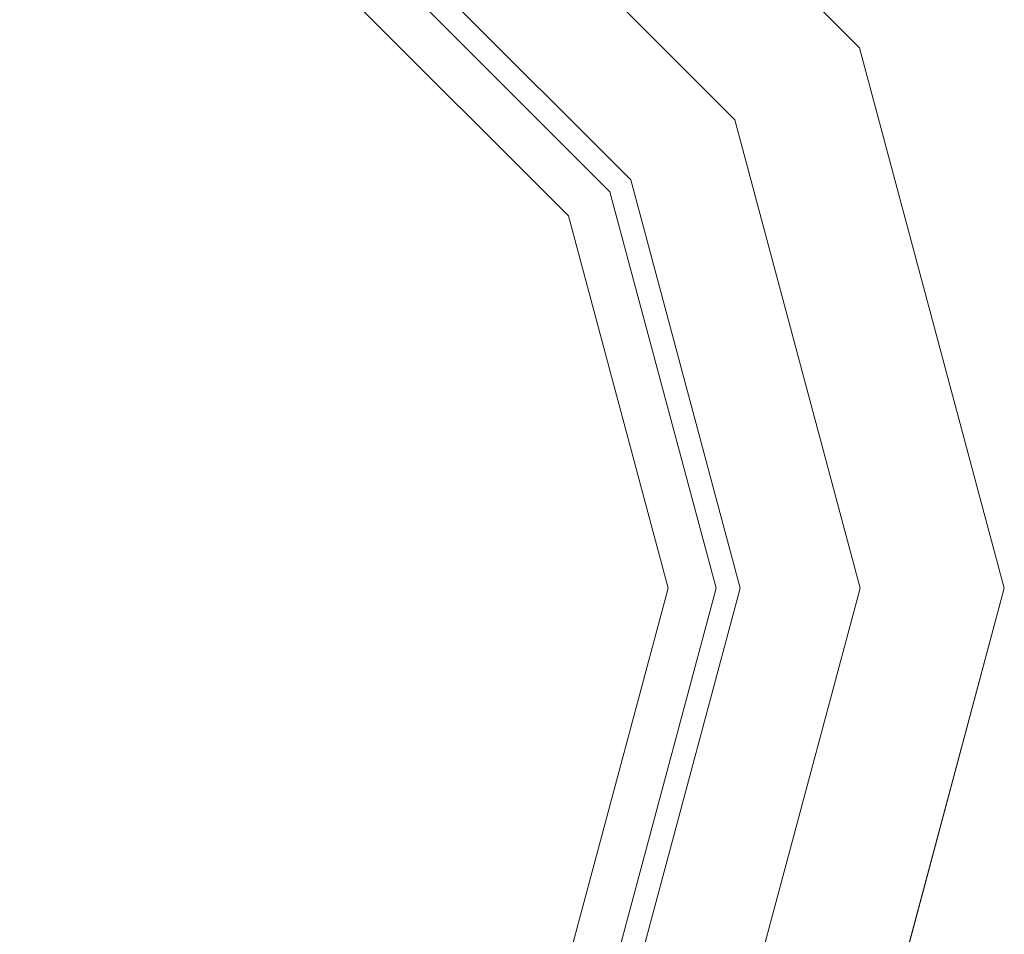
# Model space of a CAD drawing. Units: inches. Extents: x 375 to 1122, y 27 to 1069.
# Tile 24 of 155: x 713.046 to 718.094, y 275.466 to 280.154. Entities that reach past the tile are written whole.
import ezdxf

# ---------------------------------------------------------------- set-up
doc = ezdxf.new("R2010")
doc.units = ezdxf.units.IN
doc.layers.add('Furniture', color=30, linetype='Continuous', lineweight=18)

# ---------------------------------------------------------------- blocks, each defined once
blk = doc.blocks.new('A$C403C54AD')
at = {"linetype": 'ByBlock'}
for points, invisible_edges in [([(1.72651, 0.82864, -0.00874), (1.72651, 0.81017, -0.00874), (1.66648, 0.79408, -0.00874), (1.65725, 0.81008, -0.00874)], 5), ([(1.72651, 0.79478, -0.02259), (1.72651, 0.82864, -0.01335), (1.65725, 0.81008, -0.01335), (1.67418, 0.78075, -0.02259)], 5), ([(1.79578, 0.81008, -0.00874), (1.78654, 0.79408, -0.00874), (1.72651, 0.81017, -0.00874), (1.72651, 0.82864, -0.00874)], 5), ([(1.77884, 0.78075, -0.02259), (1.79578, 0.81008, -0.01335), (1.72651, 0.82864, -0.01335), (1.72651, 0.79478, -0.02259)], 5), ([(1.65725, 0.81008, -0.00874), (1.66648, 0.79408, -0.00874), (1.62254, 0.75014, -0.00874), (1.60654, 0.75938, -0.00874)], 5), ([(1.67418, 0.78075, -0.02259), (1.65725, 0.81008, -0.01335), (1.60654, 0.75938, -0.01335), (1.63587, 0.74244, -0.02259)], 5), ([(1.72651, 0.81017, -0.00874), (1.72651, 0.7917, -0.01489), (1.67572, 0.77809, -0.01489), (1.66648, 0.79408, -0.00874)], 5), ([(1.78654, 0.79408, -0.00874), (1.7773, 0.77809, -0.01489), (1.72651, 0.7917, -0.01489), (1.72651, 0.81017, -0.00874)], 5), ([(1.66648, 0.79408, -0.00874), (1.67572, 0.77809, -0.01489), (1.63853, 0.74091, -0.01489), (1.62254, 0.75014, -0.00874)], 5), ([(1.72651, 0.78554, -0.03183), (1.72651, 0.79478, -0.02259), (1.67418, 0.78075, -0.02259), (1.6788, 0.77276, -0.03183)], 5), ([(1.77423, 0.77276, -0.03183), (1.77884, 0.78075, -0.02259), (1.72651, 0.79478, -0.02259), (1.72651, 0.78554, -0.03183)], 5), ([(1.72651, 0.7917, -0.01489), (1.72651, 0.69011, -0.01489), (1.72651, 0.69011, -0.01489), (1.67572, 0.77809, -0.01489)], 5), ([(1.7773, 0.77809, -0.01489), (1.72651, 0.69011, -0.01489), (1.72651, 0.69011, -0.01489), (1.72651, 0.7917, -0.01489)], 5), ([(1.6788, 0.77276, -0.03183), (1.67418, 0.78075, -0.02259), (1.63587, 0.74244, -0.02259), (1.64387, 0.73783, -0.03183)], 1), ([(1.67572, 0.77809, -0.01489), (1.72651, 0.69011, -0.01489), (1.72651, 0.69011, -0.01489), (1.63853, 0.74091, -0.01489)], 5), ([(1.81449, 0.74091, -0.01489), (1.72651, 0.69011, -0.01489), (1.72651, 0.69011, -0.01489), (1.7773, 0.77809, -0.01489)], 5), ([(1.63853, 0.74091, -0.01489), (1.72651, 0.69011, -0.01489), (1.72651, 0.69011, -0.01489), (1.62492, 0.69011, -0.01489)], 5), ([(1.8281, 0.69011, -0.01489), (1.72651, 0.69011, -0.01489), (1.72651, 0.69011, -0.01489), (1.81449, 0.74091, -0.01489)], 5)]:
    blk.add_3dface(points, dxfattribs=dict(at, invisible_edges=invisible_edges))
for points in [[(1.72651, 0.82864, -0.01335), (1.72651, 0.82864, -0.00874), (1.65725, 0.81008, -0.00874), (1.65725, 0.81008, -0.01335)], [(1.79578, 0.81008, -0.01335), (1.79578, 0.81008, -0.00874), (1.72651, 0.82864, -0.00874), (1.72651, 0.82864, -0.01335)], [(1.65725, 0.81008, -0.01335), (1.65725, 0.81008, -0.00874), (1.60654, 0.75938, -0.00874), (1.60654, 0.75938, -0.01335)]]:
    blk.add_3dface(points, dxfattribs=at)

msp = doc.modelspace()

# ---------------------------------------------------------------- block references
at = {"layer": 'Furniture', "xscale": 39.9918517141215, "yscale": 39.9918517141215, "zscale": 39.9918517141215, "rotation": 270}
msp.add_blockref('A$C403C54AD', (684.9549, 346.2875, 0.024), dxfattribs=at)

doc.saveas('drawing.dxf')
